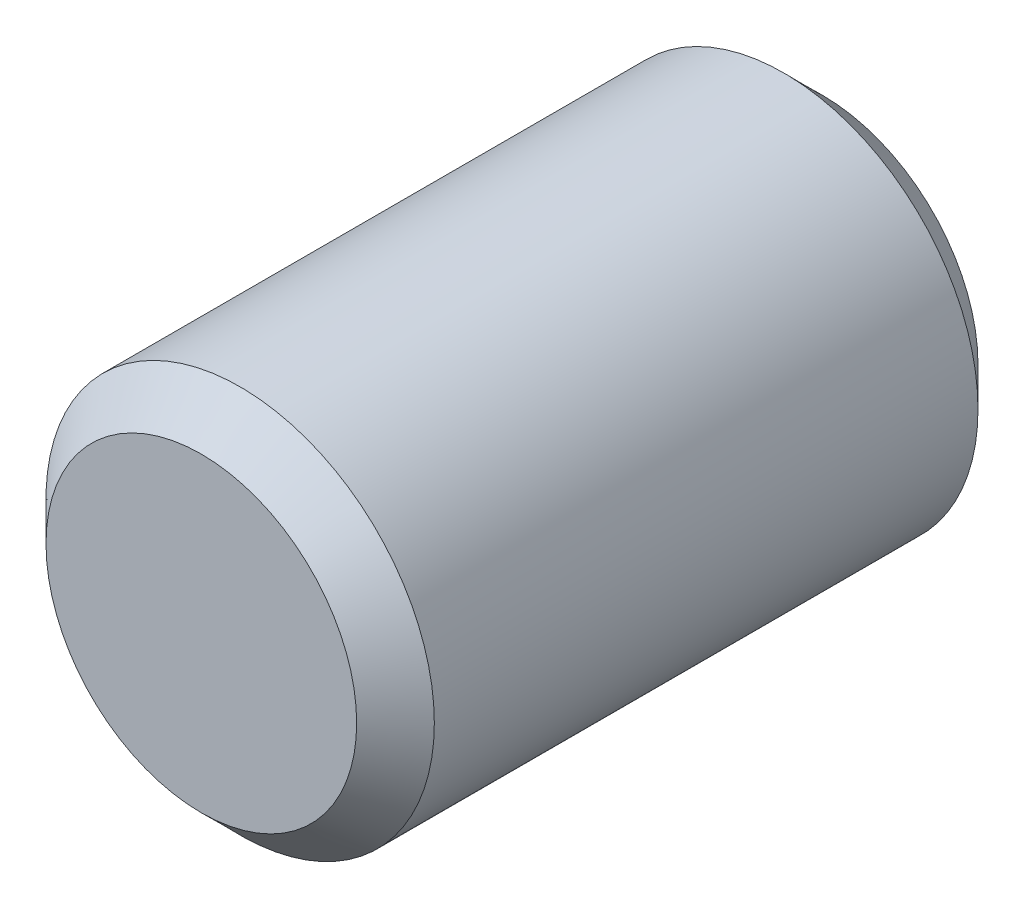
SolidWorks part; units mm, degrees
material "Plain Carbon Steel"
ref_plane "Front Plane" through (0, 0, 0) normal (0, 0, 1) x (1, 0, 0)
ref_plane "Top Plane" through (0, 0, 0) normal (0, 1, 0) x (1, 0, 0)
ref_plane "Right Plane" through (0, 0, 0) normal (1, 0, 0) x (0, 0, -1)
sketch "Pin Profile Ø5" plane through (0, 0, 0) normal (0, 0, 1) x (1, 0, 0)
  circle A0 centre (0, 0) radius 2.5
  dimension "D1" = 5
extrude "Pin Body Ø5x8" add sketch "Pin Profile Ø5" along normal blind 8
chamfer "End Chamfers 0.5x45°" distance 0.5 angle 45 2 edges at (2.5, 0, 0) (2.5, 0, 8)
